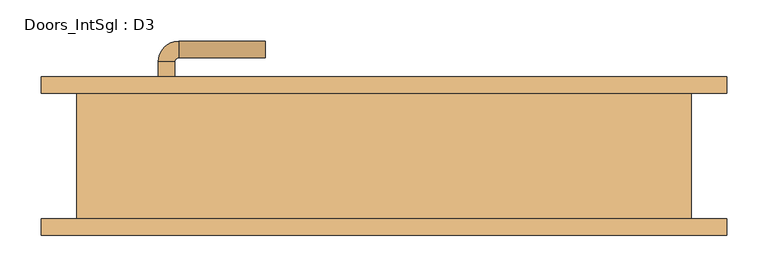
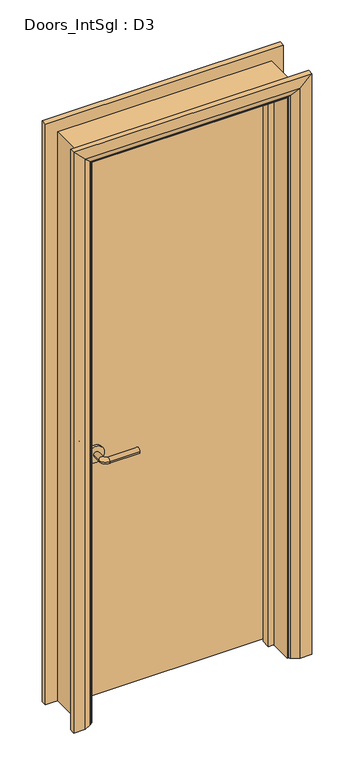
"""IFC4 building model written with IfcOpenShell, lengths in millimetres: door geometry, Doors_IntSgl : D3."""

from ifc_helpers import new_model, si_unit, point, frame, frame_2d, origin, place, context, project, spatial, polyline, circle_curve, ellipse_curve, trimmed, segment, composite_curve, outline, extrude, faceted_brep, source, transform, mapped, element, save
from ifc_brep_helpers import plane_surface, cylinder_surface, revolved_surface, advanced_brep


def doors_intsgl_d3_2a6a78d5(model_context):
    return source(origin(), model_context, "Body", "SolidModel", [
        advanced_brep(
        [(-274.0, 30.2, 900.0), (-254.0, 30.2, 900.0), (-254.0, 0.2, 900.0), (-274.0, 0.2, 900.0), (-249.0, -4.8, 900.0), (-249.0, -24.8, 900.0), (-144.0, -24.8, 900.0), (-144.0, -4.8, 900.0)],
        [
            (0, 1, circle_curve(frame((-264.0, 30.2, 900.0), z_axis=(0.0, 1.0, 0.0), x_axis=(1.0, 0.0, 0.0)), 10.0)),
            (1, 0, circle_curve(frame((-264.0, 30.2, 900.0), z_axis=(0.0, 1.0, 0.0), x_axis=(1.0, 0.0, 0.0)), 10.0)),
            (1, 2),
            (2, 3, circle_curve(frame((-264.0, 0.2, 900.0), z_axis=(0.0, 1.0, 0.0), x_axis=(1.0, 0.0, 0.0)), 10.0)),
            (3, 0),
            (3, 2, circle_curve(frame((-264.0, 0.2, 900.0), z_axis=(0.0, 1.0, 0.0), x_axis=(1.0, 0.0, 0.0)), 10.0)),
            (4, 5, circle_curve(frame((-249.0, -14.8, 900.0), z_axis=(-1.0, 0.0, 0.0), x_axis=(0.0, 1.0, 0.0)), 10.0)),
            (5, 3, circle_curve(frame((-249.0, 0.2, 900.0), z_axis=(0.0, 0.0, -1.0), x_axis=(-1.0, 0.0, 0.0)), 25.0)),
            (2, 4, circle_curve(frame((-249.0, 0.2, 900.0), z_axis=(0.0, 0.0, 1.0), x_axis=(-1.0, 0.0, 0.0)), 5.0)),
            (5, 4, circle_curve(frame((-249.0, -14.8, 900.0), z_axis=(-1.0, 0.0, 0.0), x_axis=(0.0, 1.0, 0.0)), 10.0)),
            (6, 7, circle_curve(frame((-144.0, -14.8, 900.0), z_axis=(1.0, 0.0, 0.0), x_axis=(0.0, 1.0, 0.0)), 10.0)),
            (7, 6, circle_curve(frame((-144.0, -14.8, 900.0), z_axis=(1.0, 0.0, 0.0), x_axis=(0.0, 1.0, 0.0)), 10.0)),
            (4, 7),
            (6, 5),
        ],
        [
            plane_surface(frame((-264.0, 30.2, 900.0), z_axis=(0.0, 1.0, 0.0), x_axis=(0.0, 0.0, 1.0))),
            cylinder_surface(frame((-264.0, 30.2, 900.0), z_axis=(0.0, 1.0, 0.0), x_axis=(1.0, 0.0, 0.0)), 10.0),
            revolved_surface(trimmed(ellipse_curve(frame((-264.0, 0.2, 900.0), z_axis=(0.0, -1.0, 0.0), x_axis=(1.0, 0.0, 0.0)), 10.0, 10.0), [point((-274.0, 0.2, 900.0))], [point((-254.0, 0.2, 900.0))], True, "CARTESIAN"), (-249.0, 0.2, 900.0), (0.0, 0.0, -1.0)),
            revolved_surface(trimmed(ellipse_curve(frame((-264.0, 0.2, 900.0), z_axis=(0.0, -1.0, 0.0), x_axis=(1.0, 0.0, 0.0)), 10.0, 10.0), [point((-254.0, 0.2, 900.0))], [point((-274.0, 0.2, 900.0))], True, "CARTESIAN"), (-249.0, 0.2, 900.0), (0.0, 0.0, -1.0)),
            plane_surface(frame((-144.0, -14.8, 900.0), z_axis=(1.0, 0.0, 0.0), x_axis=(0.0, 0.0, 1.0))),
            cylinder_surface(frame((-249.0, -14.8, 900.0), z_axis=(-1.0, 0.0, 0.0), x_axis=(0.0, 1.0, 0.0)), 10.0),
        ],
        [
            (0, [[1, 2]]),
            (1, [[3, 4, 5, -2]]),
            (1, [[-5, 6, -3, -1]]),
            (2, [[7, 8, -4, 9]]),
            (3, [[10, -9, -6, -8]]),
            (4, [[11, 12]]),
            (5, [[13, -11, 14, -7]]),
            (5, [[-14, -12, -13, -10]]),
        ],
    ),
        extrude(outline(composite_curve([segment(trimmed(circle_curve(frame_2d((900.0, -266.5)), 30.0), [point((900.0, -296.5))], [point((900.0, -236.5))], False, "CARTESIAN"), True, "CONTINUOUS"), segment(trimmed(circle_curve(frame_2d((900.0, -266.5)), 30.0), [point((900.0, -236.5))], [point((900.0, -296.5))], False, "CARTESIAN"), True, "CONTINUOUS")], self_intersect=False)), frame((0.0, 30.2, 0.0), z_axis=(0.0, 1.0, 0.0), x_axis=(0.0, 0.0, 1.0)), (0.0, 0.0, 1.0), 8.0),
        advanced_brep(
        [(-274.0, 84.2, 900.0), (-254.0, 84.2, 900.0), (-274.0, 114.2, 900.0), (-254.0, 114.2, 900.0), (-249.0, 119.2, 900.0), (-249.0, 139.2, 900.0), (-144.0, 139.2, 900.0), (-144.0, 119.2, 900.0)],
        [
            (0, 1, circle_curve(frame((-264.0, 84.2, 900.0), z_axis=(0.0, -1.0, 0.0), x_axis=(1.0, 0.0, 0.0)), 10.0)),
            (1, 0, circle_curve(frame((-264.0, 84.2, 900.0), z_axis=(0.0, -1.0, 0.0), x_axis=(1.0, 0.0, 0.0)), 10.0)),
            (0, 2),
            (2, 3, circle_curve(frame((-264.0, 114.2, 900.0), z_axis=(0.0, -1.0, 0.0), x_axis=(1.0, 0.0, 0.0)), 10.0)),
            (3, 1),
            (3, 2, circle_curve(frame((-264.0, 114.2, 900.0), z_axis=(0.0, -1.0, 0.0), x_axis=(1.0, 0.0, 0.0)), 10.0)),
            (4, 3, circle_curve(frame((-249.0, 114.2, 900.0), z_axis=(0.0, 0.0, 1.0), x_axis=(-1.0, 0.0, 0.0)), 5.0)),
            (2, 5, circle_curve(frame((-249.0, 114.2, 900.0), z_axis=(0.0, 0.0, -1.0), x_axis=(-1.0, 0.0, 0.0)), 25.0)),
            (5, 4, circle_curve(frame((-249.0, 129.2, 900.0), z_axis=(-1.0, 0.0, 0.0), x_axis=(0.0, -1.0, 0.0)), 10.0)),
            (4, 5, circle_curve(frame((-249.0, 129.2, 900.0), z_axis=(-1.0, 0.0, 0.0), x_axis=(0.0, -1.0, 0.0)), 10.0)),
            (6, 7, circle_curve(frame((-144.0, 129.2, 900.0), z_axis=(1.0, 0.0, 0.0), x_axis=(0.0, -1.0, 0.0)), 10.0)),
            (7, 6, circle_curve(frame((-144.0, 129.2, 900.0), z_axis=(1.0, 0.0, 0.0), x_axis=(0.0, -1.0, 0.0)), 10.0)),
            (5, 6),
            (7, 4),
        ],
        [
            plane_surface(frame((-264.0, 84.2, 900.0), z_axis=(0.0, -1.0, 0.0), x_axis=(0.0, 0.0, 1.0))),
            cylinder_surface(frame((-264.0, 84.2, 900.0), z_axis=(0.0, -1.0, 0.0), x_axis=(1.0, 0.0, 0.0)), 10.0),
            revolved_surface(trimmed(ellipse_curve(frame((-264.0, 114.2, 900.0), z_axis=(0.0, -1.0, 0.0), x_axis=(1.0, 0.0, 0.0)), 10.0, 10.0), [point((-274.0, 114.2, 900.0))], [point((-254.0, 114.2, 900.0))], True, "CARTESIAN"), (-249.0, 114.2, 900.0), (0.0, 0.0, -1.0)),
            revolved_surface(trimmed(ellipse_curve(frame((-264.0, 114.2, 900.0), z_axis=(0.0, -1.0, 0.0), x_axis=(1.0, 0.0, 0.0)), 10.0, 10.0), [point((-254.0, 114.2, 900.0))], [point((-274.0, 114.2, 900.0))], True, "CARTESIAN"), (-249.0, 114.2, 900.0), (0.0, 0.0, -1.0)),
            plane_surface(frame((-144.0, 129.2, 900.0), z_axis=(1.0, 0.0, 0.0), x_axis=(0.0, 0.0, 1.0))),
            cylinder_surface(frame((-249.0, 129.2, 900.0), z_axis=(-1.0, 0.0, 0.0), x_axis=(0.0, -1.0, 0.0)), 10.0),
        ],
        [
            (0, [[1, 2]]),
            (1, [[-1, 3, 4, 5]]),
            (1, [[-2, -5, 6, -3]]),
            (2, [[7, -4, 8, 9]]),
            (3, [[-8, -6, -7, 10]]),
            (4, [[11, 12]]),
            (5, [[-9, 13, -12, 14]]),
            (5, [[-10, -14, -11, -13]]),
        ],
    ),
        extrude(outline(composite_curve([segment(trimmed(circle_curve(frame_2d((900.0, -266.5)), 30.0), [point((900.0, -296.5))], [point((900.0, -236.5))], False, "CARTESIAN"), True, "CONTINUOUS"), segment(trimmed(circle_curve(frame_2d((900.0, -266.5)), 30.0), [point((900.0, -236.5))], [point((900.0, -296.5))], False, "CARTESIAN"), True, "CONTINUOUS")], self_intersect=False)), frame((0.0, 76.2, 0.0), z_axis=(0.0, 1.0, 0.0), x_axis=(0.0, 0.0, 1.0)), (0.0, 0.0, 1.0), 8.0),
        extrude(outline(polyline([(339.0, 38.2), (-339.0, 38.2), (-339.0, 76.2), (339.0, 76.2), (339.0, 38.2)])), frame((0.0, 0.0, 8.0), z_axis=(0.0, 0.0, 1.0), x_axis=(1.0, 0.0, 0.0)), (0.0, 0.0, 1.0), 2060.0),
        advanced_brep(
        [(416.0, 96.2, 0.0), (416.0, 76.2, 0.0), (346.0, 76.2, 0.0), (350.0, 82.2, 0.0), (376.0, 96.2, 0.0), (416.0, 96.2, 2145.0), (416.0, 76.2, 2145.0), (-416.0, 76.2, 2145.0), (-416.0, 76.2, 0.0), (-346.0, 76.2, 0.0), (-346.0, 76.2, 2075.0), (346.0, 76.2, 2075.0), (350.0, 82.2, 2079.0), (376.0, 96.2, 2105.0), (-376.0, 96.2, 2105.0), (-376.0, 96.2, 0.0), (-416.0, 96.2, 0.0), (-416.0, 96.2, 2145.0), (-350.0, 82.2, 0.0), (-350.0, 82.2, 2079.0)],
        [
            (0, 1),
            (1, 2),
            (2, 3, circle_curve(frame((354.0, 75.2, 0.0), z_axis=(0.0, 0.0, -1.0), x_axis=(1.0, 0.0, 0.0)), 8.0622577)),
            (3, 4),
            (4, 0),
            (0, 5),
            (5, 6),
            (6, 1),
            (6, 7),
            (7, 8),
            (8, 9),
            (9, 10),
            (10, 11),
            (11, 2),
            (11, 12, ellipse_curve(frame((354.0, 75.2, 2083.0), z_axis=(0.7071067811865475, 0.0, -0.7071067811865475), x_axis=(-0.7071067811865474, 0.0, -0.7071067811865476)), 11.4017543, 8.0622577)),
            (12, 3),
            (12, 13),
            (13, 4),
            (13, 14),
            (14, 15),
            (15, 16),
            (16, 17),
            (17, 5),
            (7, 17),
            (16, 8),
            (15, 18),
            (18, 9, circle_curve(frame((-354.0, 75.2, 0.0), z_axis=(0.0, 0.0, -1.0), x_axis=(-1.0, 0.0, 0.0)), 8.0622577)),
            (19, 10, ellipse_curve(frame((-354.0, 75.2, 2083.0), z_axis=(-0.7071067811865475, 0.0, -0.7071067811865475), x_axis=(-0.7071067811865474, 0.0, 0.7071067811865476)), 11.4017543, 8.0622577)),
            (18, 19),
            (14, 19),
            (19, 12),
        ],
        [
            plane_surface(frame((346.0, 76.2, 0.0), z_axis=(0.0, 0.0, -1.0), x_axis=(0.0, -1.0, 0.0))),
            plane_surface(frame((416.0, 96.2, 0.0), z_axis=(1.0, 0.0, 0.0), x_axis=(0.0, 0.0, 1.0))),
            plane_surface(frame((416.0, 76.2, 0.0), z_axis=(0.0, -1.0, 0.0), x_axis=(0.0, 0.0, 1.0))),
            cylinder_surface(frame((354.0, 75.2, 0.0), z_axis=(0.0, 0.0, -1.0), x_axis=(1.0, 0.0, 0.0)), 8.0622577),
            plane_surface(frame((350.0, 82.2, 0.0), z_axis=(-0.4740998230350126, 0.880471099922178, 0.0), x_axis=(0.0, 0.0, 1.0))),
            plane_surface(frame((376.0, 96.2, 0.0), z_axis=(0.0, 1.0, 0.0), x_axis=(0.0, 0.0, 1.0))),
            plane_surface(frame((-416.0, 96.2, 2145.0), z_axis=(-1.0, 0.0, 0.0), x_axis=(0.0, 0.0, -1.0))),
            plane_surface(frame((-346.0, 76.2, 0.0), z_axis=(0.0, 0.0, -1.0), x_axis=(0.0, -1.0, 0.0))),
            cylinder_surface(frame((-354.0, 75.2, 2075.0), z_axis=(0.0, 0.0, 1.0), x_axis=(-1.0, 0.0, 0.0)), 8.0622577),
            plane_surface(frame((-350.0, 82.2, 2079.0), z_axis=(0.47409982303501824, 0.8804710999221749, 0.0), x_axis=(0.0, 0.0, -1.0))),
            plane_surface(frame((416.0, 96.2, 2145.0), z_axis=(0.0, 0.0, 1.0), x_axis=(-1.0, 0.0, 0.0))),
            cylinder_surface(frame((346.0, 75.2, 2083.0), z_axis=(1.0, 0.0, 0.0), x_axis=(0.0, 0.0, 1.0)), 8.0622577),
            plane_surface(frame((350.0, 82.2, 2079.0), z_axis=(0.0, 0.8804710999221764, -0.4740998230350154), x_axis=(-1.0, 0.0, 0.0))),
        ],
        [
            (0, [[1, 2, 3, 4, 5]]),
            (1, [[-1, 6, 7, 8]]),
            (2, [[-2, -8, 9, 10, 11, 12, 13, 14]]),
            (3, [[-3, -14, 15, 16]]),
            (4, [[-4, -16, 17, 18]]),
            (5, [[-5, -18, 19, 20, 21, 22, 23, -6]]),
            (6, [[24, -22, 25, -10]]),
            (7, [[-21, 26, 27, -11, -25]]),
            (8, [[28, -12, -27, 29]]),
            (9, [[30, -29, -26, -20]]),
            (10, [[-7, -23, -24, -9]]),
            (11, [[-15, -13, -28, 31]]),
            (12, [[-17, -31, -30, -19]]),
        ],
    ),
        extrude(outline(polyline([(0.0, -341.0), (0.0, -322.0), (2051.0, -322.0), (2051.0, 322.0), (0.0, 322.0), (0.0, 341.0), (2070.0, 341.0), (2070.0, -341.0), (0.0, -341.0)])), frame((0.0, 4.2, 0.0), z_axis=(0.0, 1.0, 0.0), x_axis=(0.0, 0.0, 1.0)), (0.0, 0.0, 1.0), 32.0),
        advanced_brep(
        [(-416.0, -96.2, 0.0), (-416.0, -76.2, 0.0), (-346.0, -76.2, 0.0), (-350.0, -82.2, 0.0), (-376.0, -96.2, 0.0), (-416.0, -96.2, 2145.0), (-416.0, -76.2, 2145.0), (-346.0, -76.2, 2075.0), (-350.0, -82.2, 2079.0), (-376.0, -96.2, 2105.0), (416.0, -96.2, 0.0), (376.0, -96.2, 0.0), (350.0, -82.2, 0.0), (346.0, -76.2, 0.0), (416.0, -76.2, 0.0), (416.0, -96.2, 2145.0), (376.0, -96.2, 2105.0), (350.0, -82.2, 2079.0), (346.0, -76.2, 2075.0), (416.0, -76.2, 2145.0)],
        [
            (0, 1),
            (1, 2),
            (2, 3, circle_curve(frame((-354.0, -75.2, 0.0), z_axis=(0.0, 0.0, -1.0), x_axis=(-1.0, 0.0, 0.0)), 8.0622577)),
            (3, 4),
            (4, 0),
            (0, 5),
            (5, 6),
            (6, 1),
            (6, 7),
            (7, 2),
            (7, 8, ellipse_curve(frame((-354.0, -75.2, 2083.0), z_axis=(-0.7071067811865475, 0.0, -0.7071067811865475), x_axis=(0.7071067811865474, 0.0, -0.7071067811865476)), 11.4017543, 8.0622577)),
            (8, 3),
            (8, 9),
            (9, 4),
            (9, 5),
            (10, 11),
            (11, 12),
            (12, 13, circle_curve(frame((354.0, -75.2, 0.0), z_axis=(0.0, 0.0, -1.0), x_axis=(1.0, 0.0, 0.0)), 8.0622577)),
            (13, 14),
            (14, 10),
            (15, 16),
            (16, 11),
            (10, 15),
            (16, 17),
            (17, 12),
            (17, 18, ellipse_curve(frame((354.0, -75.2, 2083.0), z_axis=(0.7071067811865475, 0.0, -0.7071067811865475), x_axis=(0.7071067811865474, 0.0, 0.7071067811865476)), 11.4017543, 8.0622577)),
            (18, 13),
            (18, 19),
            (19, 14),
            (19, 15),
            (5, 15),
            (19, 6),
            (18, 7),
            (17, 8),
            (16, 9),
        ],
        [
            plane_surface(frame((-346.0, -149.0010989, 0.0), z_axis=(0.0, 0.0, -1.0), x_axis=(1.0, 0.0, 0.0))),
            plane_surface(frame((-416.0, -96.2, 0.0), z_axis=(-1.0, 0.0, 0.0), x_axis=(0.0, 0.0, 1.0))),
            plane_surface(frame((-416.0, -76.2, 0.0), z_axis=(0.0, 1.0, 0.0), x_axis=(0.0, 0.0, 1.0))),
            cylinder_surface(frame((-354.0, -75.2, 0.0), z_axis=(0.0, 0.0, -1.0), x_axis=(-1.0, 0.0, 0.0)), 8.0622577),
            plane_surface(frame((-350.0, -82.2, 0.0), z_axis=(0.4740998230350183, -0.8804710999221749, 0.0), x_axis=(0.0, 0.0, 1.0))),
            plane_surface(frame((-376.0, -96.2, 0.0), z_axis=(0.0, -1.0, 0.0), x_axis=(0.0, 0.0, 1.0))),
            plane_surface(frame((346.0, -149.0010989, 0.0), z_axis=(0.0, 0.0, -1.0), x_axis=(-1.0, 0.0, 0.0))),
            plane_surface(frame((376.0, -96.2, 2105.0), z_axis=(0.0, -1.0, 0.0), x_axis=(0.0, 0.0, -1.0))),
            plane_surface(frame((350.0, -82.2, 2079.0), z_axis=(-0.4740998230350183, -0.8804710999221749, 0.0), x_axis=(0.0, 0.0, -1.0))),
            cylinder_surface(frame((354.0, -75.2, 2075.0), z_axis=(0.0, 0.0, 1.0), x_axis=(1.0, 0.0, 0.0)), 8.0622577),
            plane_surface(frame((416.0, -76.2, 2145.0), z_axis=(0.0, 1.0, 0.0), x_axis=(0.0, 0.0, -1.0))),
            plane_surface(frame((416.0, -96.2, 2145.0), z_axis=(1.0, 0.0, 0.0), x_axis=(0.0, 0.0, -1.0))),
            plane_surface(frame((-416.0, -96.2, 2145.0), z_axis=(0.0, 0.0, 1.0), x_axis=(1.0, 0.0, 0.0))),
            plane_surface(frame((-416.0, -76.2, 2145.0), z_axis=(0.0, 1.0, 0.0), x_axis=(1.0, 0.0, 0.0))),
            cylinder_surface(frame((-346.0, -75.2, 2083.0), z_axis=(-1.0, 0.0, 0.0), x_axis=(0.0, 0.0, 1.0)), 8.0622577),
            plane_surface(frame((-350.0, -82.2, 2079.0), z_axis=(0.0, -0.8804710999221749, -0.4740998230350183), x_axis=(1.0, 0.0, 0.0))),
            plane_surface(frame((-376.0, -96.2, 2105.0), z_axis=(0.0, -1.0, 0.0), x_axis=(1.0, 0.0, 0.0))),
        ],
        [
            (0, [[1, 2, 3, 4, 5]]),
            (1, [[-1, 6, 7, 8]]),
            (2, [[-2, -8, 9, 10]]),
            (3, [[-3, -10, 11, 12]]),
            (4, [[-4, -12, 13, 14]]),
            (5, [[-5, -14, 15, -6]]),
            (6, [[16, 17, 18, 19, 20]]),
            (7, [[21, 22, -16, 23]]),
            (8, [[24, 25, -17, -22]]),
            (9, [[26, 27, -18, -25]]),
            (10, [[28, 29, -19, -27]]),
            (11, [[30, -23, -20, -29]]),
            (12, [[-7, 31, -30, 32]]),
            (13, [[-9, -32, -28, 33]]),
            (14, [[-11, -33, -26, 34]]),
            (15, [[-13, -34, -24, 35]]),
            (16, [[-15, -35, -21, -31]]),
        ],
    ),
        faceted_brep([(-341.0, 76.2, 0.0), (-341.0, -76.2, 0.0), (-373.0, -76.2, 0.0), (-373.0, 76.2, 0.0), (-341.0, 76.2, 2070.0), (-341.0, -76.2, 2070.0), (-373.0, -76.2, 2102.0), (-373.0, 76.2, 2102.0), (341.0, 76.2, 0.0), (373.0, 76.2, 0.0), (373.0, -76.2, 0.0), (341.0, -76.2, 0.0), (341.0, 76.2, 2070.0), (373.0, 76.2, 2102.0), (373.0, -76.2, 2102.0), (341.0, -76.2, 2070.0)], [[[0, 1, 2, 3]], [[1, 0, 4, 5]], [[2, 1, 5, 6]], [[3, 2, 6, 7]], [[0, 3, 7, 4]], [[8, 9, 10, 11]], [[12, 13, 9, 8]], [[13, 14, 10, 9]], [[14, 15, 11, 10]], [[15, 12, 8, 11]], [[5, 4, 12, 15]], [[6, 5, 15, 14]], [[7, 6, 14, 13]], [[4, 7, 13, 12]]]),
    ])


if __name__ == "__main__":
    model = new_model("IFC4")
    model_context = context("Model", 3, world=origin())
    ifc_project = project(units=[si_unit("LENGTHUNIT", "METRE", prefix="MILLI")], contexts=[model_context])
    site = spatial("IfcSite", under=ifc_project)
    building = spatial("IfcBuilding", under=site)
    placement = place(None, origin())
    doors_intsgl_d3_shape = doors_intsgl_d3_2a6a78d5(model_context)
    element("IfcDoor", 1, ObjectType="Doors_IntSgl : D3", at=placement, inside=building, context=model_context, shape_type="MappedRepresentation", body=[
        mapped(doors_intsgl_d3_shape, transform((0.0, 0.0, 0.0), x_axis=(1.0, 0.0, 0.0), y_axis=(0.0, 1.0, 0.0), z_axis=(0.0, 0.0, 1.0))),
    ])
    save(model, "model.ifc")

# Revit data of these elements
# Type "Doors_IntSgl : D3"
#   Type Mark = "48"
#   Type Comments = "Internal Single"
#   Operation = "SingleSwingRight"
#   Manufacturer = "Revit"
#   Keynote = "L20"
#   Description = "Internal Single Door"
#   Analytic Construction = "Metal"
#   UnderCut = 0.026247 ft
#   Tolerance = 0.006562 ft
#   Thickness = 0.124672 ft
#   Thermal Resistance (R) = 0.270117 (m²·K)/W
#   Structural Tolerance = 0.026247 ft
#   StopDepth = 0.104987 ft
#   Stop Thickness = 0.062336 ft
#   Rough Width = 2.5 ft
#   Rough Height = 6.922572 ft
#   Height to Top Lock Rail = 3.28084 ft
#   Heat Transfer Coefficient (U) = 3.7021 W/(m²·K)
#   Handle Z Distance = 2.952756 ft
#   Handle X Distance = 0.246063 ft
#   Frame Thickness = 0.104987 ft
#   Door Panel Width = 2.224409 ft
#   Door Panel Thickness = 0.124672 ft
#   Door Panel Offset = 0.0 ft
#   Height = 6.922572 ft
#   Width = 2.5 ft
#   Door Panel Height = 6.75853 ft
#   Architrave Setback = 0.016404 ft
#   Vis - Ironmongery = yes
#   Material Ironmongery = Door - Handle
#   Material Frame = Door - Frame/Mullion (1)
#   Material Door = Door - Panel
#   Material Architrave = Door - Architrave
#   Visual Light Transmittance = 0
#   Solar Heat Gain Coefficient = 0
#   Function = (empty or 0)
#   Wall Closure = (empty or 0)
# Element 1 (IfcDoor, "Doors_IntSgl : D3")
#   Materials on its faces: "Door - Architrave", "Door - Handle", "Door - Frame/Mullion (1)", "Door - Panel"
# Materials
#   "Door - Handle": colour RGB 0 0 0, transparency 0, Keynote = "P21", Cost = 0
#   "Door - Frame/Mullion (1)": class "Wood", colour RGB 212 179 113, transparency 0, Keynote = "L20", Cost = 0
#   "Door - Panel": class "Wood", colour RGB 210 159 95, transparency 0, Keynote = "L20", Cost = 0
#   "Door - Architrave": class "Wood", colour RGB 154 90 5, transparency 0, Keynote = "P20", Cost = 0
